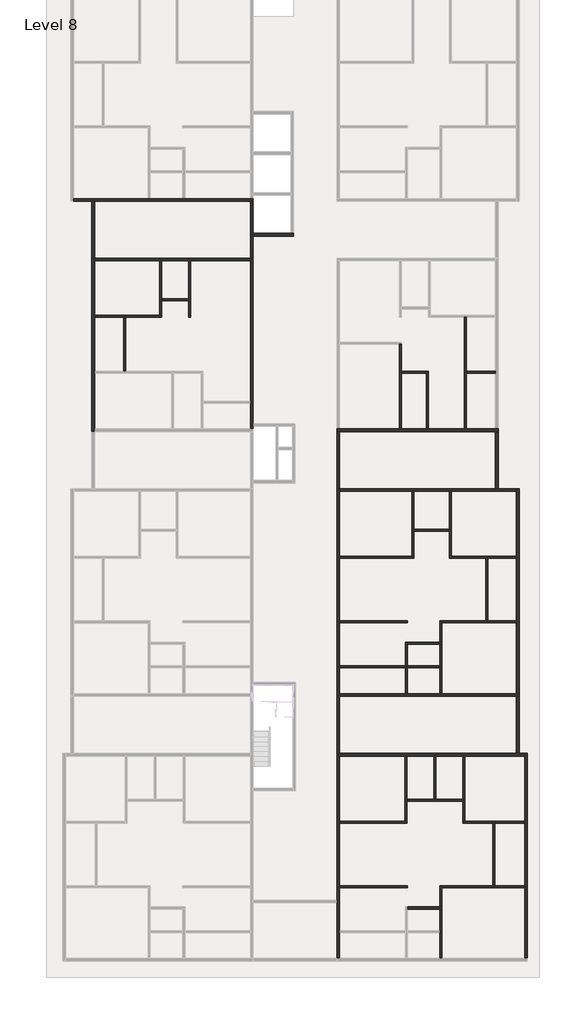
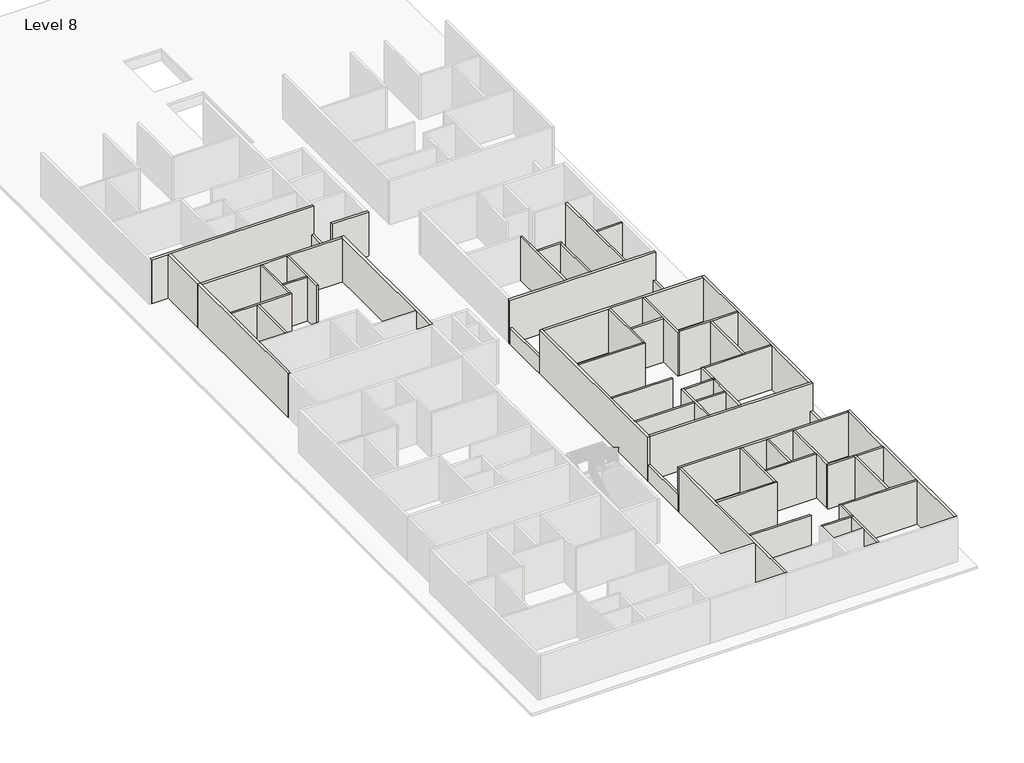
# One storey, part 2 of 8: 56 walls.
"""IFC4 building model written with IfcOpenShell, lengths in millimetres."""

from ifc_helpers import new_model, si_unit, frame, origin, place, context, project, spatial, polyline, outline, extrude, faceted_brep, element, save

model = new_model("IFC4")

# Units and contexts
model_context = context("Model", 3, world=origin())
ifc_project = project(units=[si_unit("LENGTHUNIT", "METRE", prefix="MILLI")], contexts=[model_context])

# Site, building, storey
site = spatial("IfcSite", under=ifc_project)
building = spatial("IfcBuilding", under=site)
storey = spatial("IfcBuildingStorey", under=building, Name="Level 8", Elevation=46570.6172466)

# Walls
placement = place(None, origin())
element("IfcWall", 1, ObjectType="4.5\"", at=placement, inside=storey, context=model_context, shape_type="Brep", body=[
    faceted_brep([(-12531.5544854, 2100.0216096, 46570.6172466), (-10907.2415084, 2100.0216096, 46570.6172466), (-10792.9415084, 2100.0216096, 46570.6172466), (-8759.6544854, 2100.0216096, 46570.6172466), (-8759.6544854, 2100.0216096, 49618.6172466), (-10792.9415084, 2100.0216096, 49618.6172466), (-10907.2415084, 2100.0216096, 49618.6172466), (-12531.5544854, 2100.0216096, 49618.6172466), (-12531.5544854, 2214.3216096, 46570.6172466), (-12531.5544854, 2214.3216096, 49618.6172466), (-8873.9544854, 2214.3216096, 49618.6172466), (-8759.6544854, 2214.3216096, 49618.6172466), (-8759.6544854, 2214.3216096, 46570.6172466), (-8873.9544854, 2214.3216096, 46570.6172466)], [[[0, 1, 2, 3, 4, 5, 6, 7]], [[8, 9, 10, 11, 12, 13]], [[3, 2, 1, 0, 8, 13, 12]], [[0, 7, 9, 8]], [[4, 3, 12, 11]], [[7, 6, 5, 4, 11, 10, 9]]]),
])
element("IfcWall", 2, ObjectType="4.5\"", at=placement, inside=storey, context=model_context, shape_type="Brep", body=[
    faceted_brep([(-8759.6544854, 2214.3216096, 46570.6172466), (-8759.6544854, 3014.4216096, 46570.6172466), (-8759.6544854, 3128.7216096, 46570.6172466), (-8759.6544854, 5264.2743917, 46570.6172466), (-8759.6544854, 5264.2743917, 49618.6172466), (-8759.6544854, 3128.7216096, 49618.6172466), (-8759.6544854, 3014.4216096, 49618.6172466), (-8759.6544854, 2214.3216096, 49618.6172466), (-8873.9544854, 2214.3216096, 46570.6172466), (-8873.9544854, 2214.3216096, 49618.6172466), (-8873.9544854, 5264.2743917, 49618.6172466), (-8873.9544854, 5264.2743917, 46570.6172466)], [[[0, 1, 2, 3, 4, 5, 6, 7]], [[8, 9, 10, 11]], [[3, 2, 1, 0, 8, 11]], [[0, 7, 9, 8]], [[4, 3, 11, 10]], [[7, 6, 5, 4, 10, 9]]]),
])
element("IfcWall", 3, ObjectType="4.5\"", at=placement, inside=storey, context=model_context, shape_type="Brep", body=[
    faceted_brep([(-7235.6544854, 5264.2743917, 46570.6172466), (-7235.6544854, 3128.7216096, 46570.6172466), (-7235.6544854, 3014.4216096, 46570.6172466), (-7235.6544854, 2100.0216096, 46570.6172466), (-7235.6544854, 2100.0216096, 49618.6172466), (-7235.6544854, 3014.4216096, 49618.6172466), (-7235.6544854, 3128.7216096, 49618.6172466), (-7235.6544854, 5264.2743917, 49618.6172466), (-7121.3544854, 5264.2743917, 46570.6172466), (-7121.3544854, 5264.2743917, 49618.6172466), (-7121.3544854, 2100.0216096, 49618.6172466), (-7121.3544854, 2100.0216096, 46570.6172466)], [[[0, 1, 2, 3, 4, 5, 6, 7]], [[8, 9, 10, 11]], [[3, 2, 1, 0, 8, 11]], [[4, 3, 11, 10]], [[0, 7, 9, 8]], [[7, 6, 5, 4, 10, 9]]]),
])
element("IfcWall", 4, ObjectType="4.5\"", at=placement, inside=storey, context=model_context, shape_type="SweptSolid", body=[
    extrude(outline(polyline([(-7235.6544854, 3014.4216096), (-8759.6544854, 3014.4216096), (-8759.6544854, 3128.7216096), (-7235.6544854, 3128.7216096), (-7235.6544854, 3014.4216096)])), frame((0.0, 0.0, 46570.6172466), z_axis=(0.0, 0.0, 1.0), x_axis=(1.0, 0.0, 0.0)), (0.0, 0.0, 1.0), 3048.0),
])
element("IfcWall", 5, ObjectType="4.5\"", at=placement, inside=storey, context=model_context, shape_type="SweptSolid", body=[
    extrude(outline(polyline([(-10907.2415084, -947.4344126), (-10907.2415084, 2100.0216096), (-10792.9415084, 2100.0216096), (-10792.9415084, -947.4344126), (-10907.2415084, -947.4344126)])), frame((0.0, 0.0, 46570.6172466), z_axis=(0.0, 0.0, 1.0), x_axis=(1.0, 0.0, 0.0)), (0.0, 0.0, 1.0), 3048.0),
])
element("IfcWall", 6, ObjectType="4.5\"", at=placement, inside=storey, context=model_context, shape_type="Brep", body=[
    faceted_brep([(5056.6584916, -31173.4344126, 46570.6172466), (6885.4584916, -31173.4344126, 46570.6172466), (6999.7584916, -31173.4344126, 46570.6172466), (6999.7584916, -31173.4344126, 49618.6172466), (6885.4584916, -31173.4344126, 49618.6172466), (5056.6584916, -31173.4344126, 49618.6172466), (5056.6584916, -31059.1344126, 46570.6172466), (5056.6584916, -31059.1344126, 49618.6172466), (6885.4584916, -31059.1344126, 49618.6172466), (6999.7584916, -31059.1344126, 49618.6172466), (6999.7584916, -31059.1344126, 46570.6172466), (6885.4584916, -31059.1344126, 46570.6172466)], [[[0, 1, 2, 3, 4, 5]], [[6, 7, 8, 9, 10, 11]], [[2, 1, 0, 6, 11, 10]], [[0, 5, 7, 6]], [[3, 2, 10, 9]], [[5, 4, 3, 9, 8, 7]]]),
])
element("IfcWall", 7, ObjectType="4.5\"", at=placement, inside=storey, context=model_context, shape_type="Brep", body=[
    faceted_brep([(6885.4584916, -31173.4344126, 46570.6172466), (6885.4584916, -32392.6344126, 46570.6172466), (6885.4584916, -32506.9344126, 46570.6172466), (6885.4584916, -33954.7344126, 46570.6172466), (6885.4584916, -33954.7344126, 49618.6172466), (6885.4584916, -32506.9344126, 49618.6172466), (6885.4584916, -32392.6344126, 49618.6172466), (6885.4584916, -31173.4344126, 49618.6172466), (6999.7584916, -31173.4344126, 46570.6172466), (6999.7584916, -31173.4344126, 49618.6172466), (6999.7584916, -33954.7344126, 49618.6172466), (6999.7584916, -33954.7344126, 46570.6172466)], [[[0, 1, 2, 3, 4, 5, 6, 7]], [[8, 9, 10, 11]], [[3, 2, 1, 0, 8, 11]], [[0, 7, 9, 8]], [[4, 3, 11, 10]], [[7, 6, 5, 4, 10, 9]]]),
])
element("IfcWall", 8, ObjectType="4.5\"", at=placement, inside=storey, context=model_context, shape_type="Brep", body=[
    faceted_brep([(6999.7584916, -31059.1344126, 46570.6172466), (6999.7584916, -29966.9344126, 46570.6172466), (6999.7584916, -29852.6344126, 46570.6172466), (6999.7584916, -29852.6344126, 49618.6172466), (6999.7584916, -29966.9344126, 49618.6172466), (6999.7584916, -31059.1344126, 49618.6172466), (6885.4584916, -31059.1344126, 46570.6172466), (6885.4584916, -31059.1344126, 49618.6172466), (6885.4584916, -29852.6344126, 49618.6172466), (6885.4584916, -29852.6344126, 46570.6172466)], [[[0, 1, 2, 3, 4, 5]], [[6, 7, 8, 9]], [[2, 1, 0, 6, 9]], [[0, 5, 7, 6]], [[3, 2, 9, 8]], [[5, 4, 3, 8, 7]]]),
])
element("IfcWall", 9, ObjectType="4.5\"", at=placement, inside=storey, context=model_context, shape_type="Brep", body=[
    faceted_brep([(6999.7584916, -29966.9344126, 46570.6172466), (11660.6584916, -29966.9344126, 46570.6172466), (11660.6584916, -29966.9344126, 49618.6172466), (6999.7584916, -29966.9344126, 49618.6172466), (6999.7584916, -29852.6344126, 46570.6172466), (6999.7584916, -29852.6344126, 49618.6172466), (9869.9584916, -29852.6344126, 49618.6172466), (9984.2584916, -29852.6344126, 49618.6172466), (11660.6584916, -29852.6344126, 49618.6172466), (11660.6584916, -29852.6344126, 46570.6172466), (9984.2584916, -29852.6344126, 46570.6172466), (9869.9584916, -29852.6344126, 46570.6172466)], [[[0, 1, 2, 3]], [[4, 5, 6, 7, 8, 9, 10, 11]], [[1, 0, 4, 11, 10, 9]], [[0, 3, 5, 4]], [[2, 1, 9, 8]], [[3, 2, 8, 7, 6, 5]]]),
])
element("IfcWall", 10, ObjectType="4.5\"", at=placement, inside=storey, context=model_context, shape_type="SweptSolid", body=[
    extrude(outline(polyline([(5056.6584916, -29966.9344126), (1259.3584916, -29966.9344126), (1259.3584916, -29852.6344126), (5056.6584916, -29852.6344126), (5056.6584916, -29966.9344126)])), frame((0.0, 0.0, 46570.6172466), z_axis=(0.0, 0.0, 1.0), x_axis=(1.0, 0.0, 0.0)), (0.0, 0.0, 1.0), 3048.0),
])
element("IfcWall", 11, ObjectType="4.5\"", at=placement, inside=storey, context=model_context, shape_type="Brep", body=[
    faceted_brep([(1259.3584916, -26347.4344126, 46570.6172466), (5031.2584916, -26347.4344126, 46570.6172466), (5031.2584916, -26347.4344126, 49618.6172466), (1259.3584916, -26347.4344126, 49618.6172466), (1259.3584916, -26233.1344126, 46570.6172466), (1259.3584916, -26233.1344126, 49618.6172466), (4916.9584916, -26233.1344126, 49618.6172466), (5031.2584916, -26233.1344126, 49618.6172466), (5031.2584916, -26233.1344126, 46570.6172466), (4916.9584916, -26233.1344126, 46570.6172466)], [[[0, 1, 2, 3]], [[4, 5, 6, 7, 8, 9]], [[1, 0, 4, 9, 8]], [[0, 3, 5, 4]], [[2, 1, 8, 7]], [[3, 2, 7, 6, 5]]]),
])
element("IfcWall", 12, ObjectType="4.5\"", at=placement, inside=storey, context=model_context, shape_type="Brep", body=[
    faceted_brep([(5031.2584916, -26233.1344126, 46570.6172466), (5031.2584916, -25128.2344126, 46570.6172466), (5031.2584916, -25013.9344126, 46570.6172466), (5031.2584916, -22575.5344126, 46570.6172466), (5031.2584916, -22575.5344126, 49618.6172466), (5031.2584916, -25013.9344126, 49618.6172466), (5031.2584916, -25128.2344126, 49618.6172466), (5031.2584916, -26233.1344126, 49618.6172466), (4916.9584916, -26233.1344126, 46570.6172466), (4916.9584916, -26233.1344126, 49618.6172466), (4916.9584916, -22575.5344126, 49618.6172466), (4916.9584916, -22575.5344126, 46570.6172466)], [[[0, 1, 2, 3, 4, 5, 6, 7]], [[8, 9, 10, 11]], [[3, 2, 1, 0, 8, 11]], [[0, 7, 9, 8]], [[4, 3, 11, 10]], [[7, 6, 5, 4, 10, 9]]]),
])
element("IfcWall", 13, ObjectType="4.5\"", at=placement, inside=storey, context=model_context, shape_type="Brep", body=[
    faceted_brep([(9984.2584916, -29852.6344126, 46570.6172466), (9984.2584916, -26347.4344126, 46570.6172466), (9984.2584916, -26233.1344126, 46570.6172466), (9984.2584916, -26233.1344126, 49618.6172466), (9984.2584916, -26347.4344126, 49618.6172466), (9984.2584916, -29852.6344126, 49618.6172466), (9869.9584916, -29852.6344126, 46570.6172466), (9869.9584916, -29852.6344126, 49618.6172466), (9869.9584916, -26347.4344126, 49618.6172466), (9869.9584916, -26233.1344126, 49618.6172466), (9869.9584916, -26233.1344126, 46570.6172466), (9869.9584916, -26347.4344126, 46570.6172466)], [[[0, 1, 2, 3, 4, 5]], [[6, 7, 8, 9, 10, 11]], [[2, 1, 0, 6, 11, 10]], [[0, 5, 7, 6]], [[3, 2, 10, 9]], [[5, 4, 3, 9, 8, 7]]]),
])
element("IfcWall", 14, ObjectType="4.5\"", at=placement, inside=storey, context=model_context, shape_type="SweptSolid", body=[
    extrude(outline(polyline([(11660.6584916, -26347.4344126), (9984.2584916, -26347.4344126), (9984.2584916, -26233.1344126), (11660.6584916, -26233.1344126), (11660.6584916, -26347.4344126)])), frame((0.0, 0.0, 46570.6172466), z_axis=(0.0, 0.0, 1.0), x_axis=(1.0, 0.0, 0.0)), (0.0, 0.0, 1.0), 3048.0),
])
element("IfcWall", 15, ObjectType="4.5\"", at=placement, inside=storey, context=model_context, shape_type="Brep", body=[
    faceted_brep([(9869.9584916, -26233.1344126, 46570.6172466), (8307.8584916, -26233.1344126, 46570.6172466), (8193.5584916, -26233.1344126, 46570.6172466), (8193.5584916, -26233.1344126, 49618.6172466), (8307.8584916, -26233.1344126, 49618.6172466), (9869.9584916, -26233.1344126, 49618.6172466), (9869.9584916, -26347.4344126, 46570.6172466), (9869.9584916, -26347.4344126, 49618.6172466), (8193.5584916, -26347.4344126, 49618.6172466), (8193.5584916, -26347.4344126, 46570.6172466)], [[[0, 1, 2, 3, 4, 5]], [[6, 7, 8, 9]], [[2, 1, 0, 6, 9]], [[0, 5, 7, 6]], [[3, 2, 9, 8]], [[5, 4, 3, 8, 7]]]),
])
element("IfcWall", 16, ObjectType="4.5\"", at=placement, inside=storey, context=model_context, shape_type="Brep", body=[
    faceted_brep([(8307.8584916, -26233.1344126, 46570.6172466), (8307.8584916, -22575.5344126, 46570.6172466), (8307.8584916, -22575.5344126, 49618.6172466), (8307.8584916, -26233.1344126, 49618.6172466), (8193.5584916, -26233.1344126, 46570.6172466), (8193.5584916, -26233.1344126, 49618.6172466), (8193.5584916, -25128.2344126, 49618.6172466), (8193.5584916, -25013.9344126, 49618.6172466), (8193.5584916, -22575.5344126, 49618.6172466), (8193.5584916, -22575.5344126, 46570.6172466), (8193.5584916, -25013.9344126, 46570.6172466), (8193.5584916, -25128.2344126, 46570.6172466)], [[[0, 1, 2, 3]], [[4, 5, 6, 7, 8, 9, 10, 11]], [[1, 0, 4, 11, 10, 9]], [[0, 3, 5, 4]], [[2, 1, 9, 8]], [[3, 2, 8, 7, 6, 5]]]),
])
element("IfcWall", 17, ObjectType="4.5\"", at=placement, inside=storey, context=model_context, shape_type="Brep", body=[
    faceted_brep([(5031.2584916, -25128.2344126, 46570.6172466), (8193.5584916, -25128.2344126, 46570.6172466), (8193.5584916, -25128.2344126, 49618.6172466), (5031.2584916, -25128.2344126, 49618.6172466), (5031.2584916, -25013.9344126, 46570.6172466), (5031.2584916, -25013.9344126, 49618.6172466), (6555.2584916, -25013.9344126, 49618.6172466), (6669.5584916, -25013.9344126, 49618.6172466), (8193.5584916, -25013.9344126, 49618.6172466), (8193.5584916, -25013.9344126, 46570.6172466), (6669.5584916, -25013.9344126, 46570.6172466), (6555.2584916, -25013.9344126, 46570.6172466)], [[[0, 1, 2, 3]], [[4, 5, 6, 7, 8, 9, 10, 11]], [[1, 0, 4, 11, 10, 9]], [[0, 3, 5, 4]], [[2, 1, 9, 8]], [[3, 2, 8, 7, 6, 5]]]),
])
element("IfcWall", 18, ObjectType="4.5\"", at=placement, inside=storey, context=model_context, shape_type="SweptSolid", body=[
    extrude(outline(polyline([(6555.2584916, -25013.9344126), (6555.2584916, -22575.5344126), (6669.5584916, -22575.5344126), (6669.5584916, -25013.9344126), (6555.2584916, -25013.9344126)])), frame((0.0, 0.0, 46570.6172466), z_axis=(0.0, 0.0, 1.0), x_axis=(1.0, 0.0, 0.0)), (0.0, 0.0, 1.0), 3048.0),
])
element("IfcWall", 19, ObjectType="4.5\"", at=placement, inside=storey, context=model_context, shape_type="SweptSolid", body=[
    extrude(outline(polyline([(4942.3584916, -17622.5344126), (1259.3584916, -17622.5344126), (1259.3584916, -17508.2344126), (4942.3584916, -17508.2344126), (4942.3584916, -17622.5344126)])), frame((0.0, 0.0, 46570.6172466), z_axis=(0.0, 0.0, 1.0), x_axis=(1.0, 0.0, 0.0)), (0.0, 0.0, 1.0), 3048.0),
])
element("IfcWall", 20, ObjectType="4.5\"", at=placement, inside=storey, context=model_context, shape_type="Brep", body=[
    faceted_brep([(4942.3584916, -16174.7344126, 46570.6172466), (4942.3584916, -17508.2344126, 46570.6172466), (4942.3584916, -17622.5344126, 46570.6172466), (4942.3584916, -19070.3344126, 46570.6172466), (4942.3584916, -19070.3344126, 49618.6172466), (4942.3584916, -17622.5344126, 49618.6172466), (4942.3584916, -17508.2344126, 49618.6172466), (4942.3584916, -16174.7344126, 49618.6172466), (5056.6584916, -16174.7344126, 46570.6172466), (5056.6584916, -16174.7344126, 49618.6172466), (5056.6584916, -16289.0344126, 49618.6172466), (5056.6584916, -17508.2344126, 49618.6172466), (5056.6584916, -17622.5344126, 49618.6172466), (5056.6584916, -19070.3344126, 49618.6172466), (5056.6584916, -19070.3344126, 46570.6172466), (5056.6584916, -17622.5344126, 46570.6172466), (5056.6584916, -17508.2344126, 46570.6172466), (5056.6584916, -16289.0344126, 46570.6172466)], [[[0, 1, 2, 3, 4, 5, 6, 7]], [[8, 9, 10, 11, 12, 13, 14, 15, 16, 17]], [[3, 2, 1, 0, 8, 17, 16, 15, 14]], [[4, 3, 14, 13]], [[0, 7, 9, 8]], [[7, 6, 5, 4, 13, 12, 11, 10, 9]]]),
])
element("IfcWall", 21, ObjectType="4.5\"", at=placement, inside=storey, context=model_context, shape_type="Brep", body=[
    faceted_brep([(5056.6584916, -16289.0344126, 46570.6172466), (6885.4584916, -16289.0344126, 46570.6172466), (6999.7584916, -16289.0344126, 46570.6172466), (6999.7584916, -16289.0344126, 49618.6172466), (6885.4584916, -16289.0344126, 49618.6172466), (5056.6584916, -16289.0344126, 49618.6172466), (5056.6584916, -16174.7344126, 46570.6172466), (5056.6584916, -16174.7344126, 49618.6172466), (6885.4584916, -16174.7344126, 49618.6172466), (6999.7584916, -16174.7344126, 49618.6172466), (6999.7584916, -16174.7344126, 46570.6172466), (6885.4584916, -16174.7344126, 46570.6172466)], [[[0, 1, 2, 3, 4, 5]], [[6, 7, 8, 9, 10, 11]], [[2, 1, 0, 6, 11, 10]], [[0, 5, 7, 6]], [[3, 2, 10, 9]], [[5, 4, 3, 9, 8, 7]]]),
])
element("IfcWall", 22, ObjectType="4.5\"", at=placement, inside=storey, context=model_context, shape_type="Brep", body=[
    faceted_brep([(6885.4584916, -16289.0344126, 46570.6172466), (6885.4584916, -17508.2344126, 46570.6172466), (6885.4584916, -17622.5344126, 46570.6172466), (6885.4584916, -19070.3344126, 46570.6172466), (6885.4584916, -19070.3344126, 49618.6172466), (6885.4584916, -17622.5344126, 49618.6172466), (6885.4584916, -17508.2344126, 49618.6172466), (6885.4584916, -16289.0344126, 49618.6172466), (6999.7584916, -16289.0344126, 46570.6172466), (6999.7584916, -16289.0344126, 49618.6172466), (6999.7584916, -19070.3344126, 49618.6172466), (6999.7584916, -19070.3344126, 46570.6172466)], [[[0, 1, 2, 3, 4, 5, 6, 7]], [[8, 9, 10, 11]], [[3, 2, 1, 0, 8, 11]], [[0, 7, 9, 8]], [[4, 3, 11, 10]], [[7, 6, 5, 4, 10, 9]]]),
])
element("IfcWall", 23, ObjectType="4.5\"", at=placement, inside=storey, context=model_context, shape_type="SweptSolid", body=[
    extrude(outline(polyline([(6885.4584916, -17622.5344126), (5056.6584916, -17622.5344126), (5056.6584916, -17508.2344126), (6885.4584916, -17508.2344126), (6885.4584916, -17622.5344126)])), frame((0.0, 0.0, 46570.6172466), z_axis=(0.0, 0.0, 1.0), x_axis=(1.0, 0.0, 0.0)), (0.0, 0.0, 1.0), 3048.0),
])
element("IfcWall", 24, ObjectType="4.5\"", at=placement, inside=storey, context=model_context, shape_type="Brep", body=[
    faceted_brep([(6999.7584916, -16174.7344126, 46570.6172466), (6999.7584916, -15082.5344126, 46570.6172466), (6999.7584916, -14968.2344126, 46570.6172466), (6999.7584916, -14968.2344126, 49618.6172466), (6999.7584916, -15082.5344126, 49618.6172466), (6999.7584916, -16174.7344126, 49618.6172466), (6885.4584916, -16174.7344126, 46570.6172466), (6885.4584916, -16174.7344126, 49618.6172466), (6885.4584916, -14968.2344126, 49618.6172466), (6885.4584916, -14968.2344126, 46570.6172466)], [[[0, 1, 2, 3, 4, 5]], [[6, 7, 8, 9]], [[2, 1, 0, 6, 9]], [[0, 5, 7, 6]], [[3, 2, 9, 8]], [[5, 4, 3, 8, 7]]]),
])
element("IfcWall", 25, ObjectType="4.5\"", at=placement, inside=storey, context=model_context, shape_type="Brep", body=[
    faceted_brep([(6999.7584916, -15082.5344126, 46570.6172466), (11208.5214687, -15082.5344126, 46570.6172466), (11208.5214687, -15082.5344126, 49618.6172466), (6999.7584916, -15082.5344126, 49618.6172466), (6999.7584916, -14968.2344126, 46570.6172466), (6999.7584916, -14968.2344126, 49618.6172466), (9469.9084916, -14968.2344126, 49618.6172466), (9584.2084916, -14968.2344126, 49618.6172466), (11208.5214687, -14968.2344126, 49618.6172466), (11208.5214687, -14968.2344126, 46570.6172466), (9584.2084916, -14968.2344126, 46570.6172466), (9469.9084916, -14968.2344126, 46570.6172466)], [[[0, 1, 2, 3]], [[4, 5, 6, 7, 8, 9, 10, 11]], [[1, 0, 4, 11, 10, 9]], [[0, 3, 5, 4]], [[2, 1, 9, 8]], [[3, 2, 8, 7, 6, 5]]]),
])
element("IfcWall", 26, ObjectType="4.5\"", at=placement, inside=storey, context=model_context, shape_type="SweptSolid", body=[
    extrude(outline(polyline([(5056.6584916, -15082.5344126), (1259.3584916, -15082.5344126), (1259.3584916, -14968.2344126), (5056.6584916, -14968.2344126), (5056.6584916, -15082.5344126)])), frame((0.0, 0.0, 46570.6172466), z_axis=(0.0, 0.0, 1.0), x_axis=(1.0, 0.0, 0.0)), (0.0, 0.0, 1.0), 3048.0),
])
element("IfcWall", 27, ObjectType="4.5\"", at=placement, inside=storey, context=model_context, shape_type="Brep", body=[
    faceted_brep([(1259.3584916, -11463.0344126, 46570.6172466), (5430.0214687, -11463.0344126, 46570.6172466), (5430.0214687, -11463.0344126, 49618.6172466), (1259.3584916, -11463.0344126, 49618.6172466), (1259.3584916, -11348.7344126, 46570.6172466), (1259.3584916, -11348.7344126, 49618.6172466), (5315.7214687, -11348.7344126, 49618.6172466), (5430.0214687, -11348.7344126, 49618.6172466), (5430.0214687, -11348.7344126, 46570.6172466), (5315.7214687, -11348.7344126, 46570.6172466)], [[[0, 1, 2, 3]], [[4, 5, 6, 7, 8, 9]], [[1, 0, 4, 9, 8]], [[0, 3, 5, 4]], [[2, 1, 8, 7]], [[3, 2, 7, 6, 5]]]),
])
element("IfcWall", 28, ObjectType="4.5\"", at=placement, inside=storey, context=model_context, shape_type="Brep", body=[
    faceted_brep([(5430.0214687, -11348.7344126, 46570.6172466), (5430.0214687, -9939.0344126, 46570.6172466), (5430.0214687, -9824.7344126, 46570.6172466), (5430.0214687, -7691.1344126, 46570.6172466), (5430.0214687, -7691.1344126, 49618.6172466), (5430.0214687, -9824.7344126, 49618.6172466), (5430.0214687, -9939.0344126, 49618.6172466), (5430.0214687, -11348.7344126, 49618.6172466), (5315.7214687, -11348.7344126, 46570.6172466), (5315.7214687, -11348.7344126, 49618.6172466), (5315.7214687, -7691.1344126, 49618.6172466), (5315.7214687, -7691.1344126, 46570.6172466)], [[[0, 1, 2, 3, 4, 5, 6, 7]], [[8, 9, 10, 11]], [[3, 2, 1, 0, 8, 11]], [[0, 7, 9, 8]], [[4, 3, 11, 10]], [[7, 6, 5, 4, 10, 9]]]),
])
element("IfcWall", 29, ObjectType="4.5\"", at=placement, inside=storey, context=model_context, shape_type="SweptSolid", body=[
    extrude(outline(polyline([(7436.6214687, -9939.0344126), (5430.0214687, -9939.0344126), (5430.0214687, -9824.7344126), (7436.6214687, -9824.7344126), (7436.6214687, -9939.0344126)])), frame((0.0, 0.0, 46570.6172466), z_axis=(0.0, 0.0, 1.0), x_axis=(1.0, 0.0, 0.0)), (0.0, 0.0, 1.0), 3048.0),
])
element("IfcWall", 30, ObjectType="4.5\"", at=placement, inside=storey, context=model_context, shape_type="Brep", body=[
    faceted_brep([(7436.6214687, -7691.1344126, 46570.6172466), (7436.6214687, -9824.7344126, 46570.6172466), (7436.6214687, -9939.0344126, 46570.6172466), (7436.6214687, -11463.0344126, 46570.6172466), (7436.6214687, -11463.0344126, 49618.6172466), (7436.6214687, -9939.0344126, 49618.6172466), (7436.6214687, -9824.7344126, 49618.6172466), (7436.6214687, -7691.1344126, 49618.6172466), (7550.9214687, -7691.1344126, 46570.6172466), (7550.9214687, -7691.1344126, 49618.6172466), (7550.9214687, -11348.7344126, 49618.6172466), (7550.9214687, -11463.0344126, 49618.6172466), (7550.9214687, -11463.0344126, 46570.6172466), (7550.9214687, -11348.7344126, 46570.6172466)], [[[0, 1, 2, 3, 4, 5, 6, 7]], [[8, 9, 10, 11, 12, 13]], [[3, 2, 1, 0, 8, 13, 12]], [[0, 7, 9, 8]], [[4, 3, 12, 11]], [[7, 6, 5, 4, 11, 10, 9]]]),
])
element("IfcWall", 31, ObjectType="4.5\"", at=placement, inside=storey, context=model_context, shape_type="Brep", body=[
    faceted_brep([(7550.9214687, -11463.0344126, 46570.6172466), (9469.9084916, -11463.0344126, 46570.6172466), (9584.2084916, -11463.0344126, 46570.6172466), (11208.5214687, -11463.0344126, 46570.6172466), (11208.5214687, -11463.0344126, 49618.6172466), (9584.2084916, -11463.0344126, 49618.6172466), (9469.9084916, -11463.0344126, 49618.6172466), (7550.9214687, -11463.0344126, 49618.6172466), (7550.9214687, -11348.7344126, 46570.6172466), (7550.9214687, -11348.7344126, 49618.6172466), (11208.5214687, -11348.7344126, 49618.6172466), (11208.5214687, -11348.7344126, 46570.6172466)], [[[0, 1, 2, 3, 4, 5, 6, 7]], [[8, 9, 10, 11]], [[3, 2, 1, 0, 8, 11]], [[0, 7, 9, 8]], [[4, 3, 11, 10]], [[7, 6, 5, 4, 10, 9]]]),
])
element("IfcWall", 32, ObjectType="4.5\"", at=placement, inside=storey, context=model_context, shape_type="SweptSolid", body=[
    extrude(outline(polyline([(9469.9084916, -14968.2344126), (9469.9084916, -11463.0344126), (9584.2084916, -11463.0344126), (9584.2084916, -14968.2344126), (9469.9084916, -14968.2344126)])), frame((0.0, 0.0, 46570.6172466), z_axis=(0.0, 0.0, 1.0), x_axis=(1.0, 0.0, 0.0)), (0.0, 0.0, 1.0), 3048.0),
])
element("IfcWall", 33, ObjectType="4.5\"", at=placement, inside=storey, context=model_context, shape_type="Brep", body=[
    faceted_brep([(4610.8714687, 572.7745083, 46570.6172466), (4610.8714687, -4185.9344126, 46570.6172466), (4610.8714687, -4185.9344126, 49618.6172466), (4610.8714687, 572.7745083, 49618.6172466), (4725.1714687, 572.7745083, 46570.6172466), (4725.1714687, 572.7745083, 49618.6172466), (4725.1714687, -947.4344126, 49618.6172466), (4725.1714687, -1061.7344126, 49618.6172466), (4725.1714687, -4185.9344126, 49618.6172466), (4725.1714687, -4185.9344126, 46570.6172466), (4725.1714687, -1061.7344126, 46570.6172466), (4725.1714687, -947.4344126, 46570.6172466)], [[[0, 1, 2, 3]], [[4, 5, 6, 7, 8, 9, 10, 11]], [[1, 0, 4, 11, 10, 9]], [[0, 3, 5, 4]], [[2, 1, 9, 8]], [[3, 2, 8, 7, 6, 5]]]),
])
element("IfcWall", 34, ObjectType="4.5\"", at=placement, inside=storey, context=model_context, shape_type="Brep", body=[
    faceted_brep([(4725.1714687, -1061.7344126, 46570.6172466), (6134.8714687, -1061.7344126, 46570.6172466), (6249.1714687, -1061.7344126, 46570.6172466), (6249.1714687, -1061.7344126, 49618.6172466), (6134.8714687, -1061.7344126, 49618.6172466), (4725.1714687, -1061.7344126, 49618.6172466), (4725.1714687, -947.4344126, 46570.6172466), (4725.1714687, -947.4344126, 49618.6172466), (6249.1714687, -947.4344126, 49618.6172466), (6249.1714687, -947.4344126, 46570.6172466)], [[[0, 1, 2, 3, 4, 5]], [[6, 7, 8, 9]], [[2, 1, 0, 6, 9]], [[0, 5, 7, 6]], [[3, 2, 9, 8]], [[5, 4, 3, 8, 7]]]),
])
element("IfcWall", 35, ObjectType="4.5\"", at=placement, inside=storey, context=model_context, shape_type="SweptSolid", body=[
    extrude(outline(polyline([(6134.8714687, -4185.9344126), (6134.8714687, -1061.7344126), (6249.1714687, -1061.7344126), (6249.1714687, -4185.9344126), (6134.8714687, -4185.9344126)])), frame((0.0, 0.0, 46570.6172466), z_axis=(0.0, 0.0, 1.0), x_axis=(1.0, 0.0, 0.0)), (0.0, 0.0, 1.0), 3048.0),
])
element("IfcWall", 36, ObjectType="4.5\"", at=placement, inside=storey, context=model_context, shape_type="Brep", body=[
    faceted_brep([(8396.7584916, -4185.9344126, 46570.6172466), (8396.7584916, -1061.7344126, 46570.6172466), (8396.7584916, -947.4344126, 46570.6172466), (8396.7584916, 2100.0216096, 46570.6172466), (8396.7584916, 2100.0216096, 49618.6172466), (8396.7584916, -947.4344126, 49618.6172466), (8396.7584916, -1061.7344126, 49618.6172466), (8396.7584916, -4185.9344126, 49618.6172466), (8282.4584916, -4185.9344126, 46570.6172466), (8282.4584916, -4185.9344126, 49618.6172466), (8282.4584916, 2100.0216096, 49618.6172466), (8282.4584916, 2100.0216096, 46570.6172466)], [[[0, 1, 2, 3, 4, 5, 6, 7]], [[8, 9, 10, 11]], [[3, 2, 1, 0, 8, 11]], [[0, 7, 9, 8]], [[4, 3, 11, 10]], [[7, 6, 5, 4, 10, 9]]]),
])
element("IfcWall", 37, ObjectType="4.5\"", at=placement, inside=storey, context=model_context, shape_type="SweptSolid", body=[
    extrude(outline(polyline([(8396.7584916, -947.4344126), (10021.0714687, -947.4344126), (10021.0714687, -1061.7344126), (8396.7584916, -1061.7344126), (8396.7584916, -947.4344126)])), frame((0.0, 0.0, 46570.6172466), z_axis=(0.0, 0.0, 1.0), x_axis=(1.0, 0.0, 0.0)), (0.0, 0.0, 1.0), 3048.0),
])
element("IfcWall", 38, ObjectType="6\"", at=placement, inside=storey, context=model_context, shape_type="Brep", body=[
    faceted_brep([(-13719.0044854, 8615.1216096, 46570.6172466), (-12683.9544854, 8615.1216096, 46570.6172466), (-12531.5544854, 8615.1216096, 46570.6172466), (-3769.8415084, 8615.1216096, 46570.6172466), (-3617.4415084, 8615.1216096, 46570.6172466), (-3617.4415084, 8615.1216096, 47789.8172466), (-3617.4415084, 8615.1216096, 49618.6172466), (-12531.5544854, 8615.1216096, 49618.6172466), (-12683.9544854, 8615.1216096, 49618.6172466), (-13719.0044854, 8615.1216096, 49618.6172466), (-13719.0044854, 8767.5216096, 46570.6172466), (-13719.0044854, 8767.5216096, 49618.6172466), (-9510.2415084, 8767.5216096, 49618.6172466), (-9395.9415084, 8767.5216096, 49618.6172466), (-7567.1415084, 8767.5216096, 49618.6172466), (-7452.8415084, 8767.5216096, 49618.6172466), (-3769.8415084, 8767.5216096, 49618.6172466), (-3617.4415084, 8767.5216096, 49618.6172466), (-3617.4415084, 8767.5216096, 46570.6172466), (-3769.8415084, 8767.5216096, 46570.6172466), (-7452.8415084, 8767.5216096, 46570.6172466), (-7567.1415084, 8767.5216096, 46570.6172466), (-9395.9415084, 8767.5216096, 46570.6172466), (-9510.2415084, 8767.5216096, 46570.6172466)], [[[0, 1, 2, 3, 4, 5, 6, 7, 8, 9]], [[10, 11, 12, 13, 14, 15, 16, 17, 18, 19, 20, 21, 22, 23]], [[4, 3, 2, 1, 0, 10, 23, 22, 21, 20, 19, 18]], [[0, 9, 11, 10]], [[4, 18, 17, 6, 5]], [[9, 8, 7, 6, 17, 16, 15, 14, 13, 12, 11]]]),
])
element("IfcWall", 39, ObjectType="6\"", at=placement, inside=storey, context=model_context, shape_type="Brep", body=[
    faceted_brep([(-12683.9544854, 5416.6743917, 46570.6172466), (-12683.9544854, -4338.3344126, 46570.6172466), (-12683.9544854, -4338.3344126, 49618.6172466), (-12683.9544854, 5416.6743917, 49618.6172466), (-12531.5544854, 5416.6743917, 46570.6172466), (-12531.5544854, 5416.6743917, 49618.6172466), (-12531.5544854, 5264.2743917, 49618.6172466), (-12531.5544854, 2214.3216096, 49618.6172466), (-12531.5544854, 2100.0216096, 49618.6172466), (-12531.5544854, -947.4344126, 49618.6172466), (-12531.5544854, -1061.7344126, 49618.6172466), (-12531.5544854, -4185.9344126, 49618.6172466), (-12531.5544854, -4338.3344126, 49618.6172466), (-12531.5544854, -4338.3344126, 46570.6172466), (-12531.5544854, -4185.9344126, 46570.6172466), (-12531.5544854, -1061.7344126, 46570.6172466), (-12531.5544854, -947.4344126, 46570.6172466), (-12531.5544854, 2100.0216096, 46570.6172466), (-12531.5544854, 2214.3216096, 46570.6172466), (-12531.5544854, 5264.2743917, 46570.6172466)], [[[0, 1, 2, 3]], [[4, 5, 6, 7, 8, 9, 10, 11, 12, 13, 14, 15, 16, 17, 18, 19]], [[1, 0, 4, 19, 18, 17, 16, 15, 14, 13]], [[2, 1, 13, 12]], [[0, 3, 5, 4]], [[3, 2, 12, 11, 10, 9, 8, 7, 6, 5]]]),
])
element("IfcWall", 40, ObjectType="6\"", at=placement, inside=storey, context=model_context, shape_type="Brep", body=[
    faceted_brep([(-3617.4415084, -4185.9344126, 46570.6172466), (-3617.4415084, -4034.6751812, 46570.6172466), (-3617.4415084, -3882.2751812, 46570.6172466), (-3617.4415084, 5416.6743917, 46570.6172466), (-3617.4415084, 5416.6743917, 49618.6172466), (-3617.4415084, -3882.2751812, 49618.6172466), (-3617.4415084, -4034.6751812, 49618.6172466), (-3617.4415084, -4185.9344126, 49618.6172466), (-3769.8415084, -4185.9344126, 46570.6172466), (-3769.8415084, -4185.9344126, 49618.6172466), (-3769.8415084, -2738.1344126, 49618.6172466), (-3769.8415084, -2623.8344126, 49618.6172466), (-3769.8415084, 5264.2743917, 49618.6172466), (-3769.8415084, 5416.6743917, 49618.6172466), (-3769.8415084, 5416.6743917, 46570.6172466), (-3769.8415084, 5264.2743917, 46570.6172466), (-3769.8415084, -2623.8344126, 46570.6172466), (-3769.8415084, -2738.1344126, 46570.6172466)], [[[0, 1, 2, 3, 4, 5, 6, 7]], [[8, 9, 10, 11, 12, 13, 14, 15, 16, 17]], [[3, 2, 1, 0, 8, 17, 16, 15, 14]], [[0, 7, 9, 8]], [[3, 14, 13, 4]], [[7, 6, 5, 4, 13, 12, 11, 10, 9]]]),
])
element("IfcWall", 41, ObjectType="6\"", at=placement, inside=storey, context=model_context, shape_type="Brep", body=[
    faceted_brep([(-3769.8415084, 5416.6743917, 49618.6172466), (-3769.8415084, 5416.6743917, 46570.6172466), (-12531.5544854, 5416.6743917, 46570.6172466), (-12531.5544854, 5416.6743917, 49618.6172466), (-3769.8415084, 5264.2743917, 46570.6172466), (-3769.8415084, 5264.2743917, 49618.6172466), (-7121.3544854, 5264.2743917, 49618.6172466), (-7235.6544854, 5264.2743917, 49618.6172466), (-8759.6544854, 5264.2743917, 49618.6172466), (-8873.9544854, 5264.2743917, 49618.6172466), (-12531.5544854, 5264.2743917, 49618.6172466), (-12531.5544854, 5264.2743917, 46570.6172466), (-8873.9544854, 5264.2743917, 46570.6172466), (-8759.6544854, 5264.2743917, 46570.6172466), (-7235.6544854, 5264.2743917, 46570.6172466), (-7121.3544854, 5264.2743917, 46570.6172466)], [[[0, 1, 2, 3]], [[4, 5, 6, 7, 8, 9, 10, 11, 12, 13, 14, 15]], [[2, 1, 4, 15, 14, 13, 12, 11]], [[3, 2, 11, 10]], [[0, 5, 4, 1]], [[0, 3, 10, 9, 8, 7, 6, 5]]]),
])
element("IfcWall", 42, ObjectType="6\"", at=placement, inside=storey, context=model_context, shape_type="Brep", body=[
    faceted_brep([(11813.0584916, -33954.7344126, 46570.6172466), (11813.0584916, -22423.1344126, 46570.6172466), (11813.0584916, -22423.1344126, 49618.6172466), (11813.0584916, -33954.7344126, 49618.6172466), (11660.6584916, -33954.7344126, 46570.6172466), (11660.6584916, -33954.7344126, 49618.6172466), (11660.6584916, -29966.9344126, 49618.6172466), (11660.6584916, -29852.6344126, 49618.6172466), (11660.6584916, -26347.4344126, 49618.6172466), (11660.6584916, -26233.1344126, 49618.6172466), (11660.6584916, -22575.5344126, 49618.6172466), (11660.6584916, -22423.1344126, 49618.6172466), (11660.6584916, -22423.1344126, 46570.6172466), (11660.6584916, -22575.5344126, 46570.6172466), (11660.6584916, -26233.1344126, 46570.6172466), (11660.6584916, -26347.4344126, 46570.6172466), (11660.6584916, -29852.6344126, 46570.6172466), (11660.6584916, -29966.9344126, 46570.6172466)], [[[0, 1, 2, 3]], [[4, 5, 6, 7, 8, 9, 10, 11, 12, 13, 14, 15, 16, 17]], [[1, 0, 4, 17, 16, 15, 14, 13, 12]], [[0, 3, 5, 4]], [[2, 1, 12, 11]], [[3, 2, 11, 10, 9, 8, 7, 6, 5]]]),
])
element("IfcWall", 43, ObjectType="6\"", at=placement, inside=storey, context=model_context, shape_type="Brep", body=[
    faceted_brep([(11660.6584916, -22423.1344126, 46570.6172466), (11360.9214687, -22423.1344126, 46570.6172466), (11208.5214687, -22423.1344126, 46570.6172466), (1259.3584916, -22423.1344126, 46570.6172466), (1106.9584916, -22423.1344126, 46570.6172466), (1106.9584916, -22423.1344126, 47789.8172466), (1106.9584916, -22423.1344126, 49618.6172466), (11660.6584916, -22423.1344126, 49618.6172466), (11660.6584916, -22575.5344126, 46570.6172466), (11660.6584916, -22575.5344126, 49618.6172466), (8307.8584916, -22575.5344126, 49618.6172466), (8193.5584916, -22575.5344126, 49618.6172466), (6669.5584916, -22575.5344126, 49618.6172466), (6555.2584916, -22575.5344126, 49618.6172466), (5031.2584916, -22575.5344126, 49618.6172466), (4916.9584916, -22575.5344126, 49618.6172466), (1259.3584916, -22575.5344126, 49618.6172466), (1106.9584916, -22575.5344126, 49618.6172466), (1106.9584916, -22575.5344126, 46570.6172466), (1259.3584916, -22575.5344126, 46570.6172466), (4916.9584916, -22575.5344126, 46570.6172466), (5031.2584916, -22575.5344126, 46570.6172466), (6555.2584916, -22575.5344126, 46570.6172466), (6669.5584916, -22575.5344126, 46570.6172466), (8193.5584916, -22575.5344126, 46570.6172466), (8307.8584916, -22575.5344126, 46570.6172466)], [[[0, 1, 2, 3, 4, 5, 6, 7]], [[8, 9, 10, 11, 12, 13, 14, 15, 16, 17, 18, 19, 20, 21, 22, 23, 24, 25]], [[4, 3, 2, 1, 0, 8, 25, 24, 23, 22, 21, 20, 19, 18]], [[0, 7, 9, 8]], [[4, 18, 17, 6, 5]], [[7, 6, 17, 16, 15, 14, 13, 12, 11, 10, 9]]]),
])
element("IfcWall", 44, ObjectType="6\"", at=placement, inside=storey, context=model_context, shape_type="Brep", body=[
    faceted_brep([(1106.9584916, -22575.5344126, 49618.6172466), (1106.9584916, -22575.5344126, 46570.6172466), (1106.9584916, -30668.5325185, 46570.6172466), (1106.9584916, -30820.9325185, 46570.6172466), (1106.9584916, -33954.7344126, 46570.6172466), (1106.9584916, -33954.7344126, 49618.6172466), (1106.9584916, -30820.9325185, 49618.6172466), (1106.9584916, -30668.5325185, 49618.6172466), (1259.3584916, -22575.5344126, 46570.6172466), (1259.3584916, -22575.5344126, 49618.6172466), (1259.3584916, -26233.1344126, 49618.6172466), (1259.3584916, -26347.4344126, 49618.6172466), (1259.3584916, -29852.6344126, 49618.6172466), (1259.3584916, -29966.9344126, 49618.6172466), (1259.3584916, -32392.6344126, 49618.6172466), (1259.3584916, -32506.9344126, 49618.6172466), (1259.3584916, -33954.7344126, 49618.6172466), (1259.3584916, -33954.7344126, 46570.6172466), (1259.3584916, -32506.9344126, 46570.6172466), (1259.3584916, -32392.6344126, 46570.6172466), (1259.3584916, -29966.9344126, 46570.6172466), (1259.3584916, -29852.6344126, 46570.6172466), (1259.3584916, -26347.4344126, 46570.6172466), (1259.3584916, -26233.1344126, 46570.6172466)], [[[0, 1, 2, 3, 4, 5, 6, 7]], [[8, 9, 10, 11, 12, 13, 14, 15, 16, 17, 18, 19, 20, 21, 22, 23]], [[4, 3, 2, 1, 8, 23, 22, 21, 20, 19, 18, 17]], [[5, 4, 17, 16]], [[0, 9, 8, 1]], [[0, 7, 6, 5, 16, 15, 14, 13, 12, 11, 10, 9]]]),
])
element("IfcWall", 45, ObjectType="6\"", at=placement, inside=storey, context=model_context, shape_type="Brep", body=[
    faceted_brep([(1106.9584916, -7538.7344126, 49618.6172466), (1106.9584916, -7538.7344126, 46570.6172466), (1106.9584916, -19222.7344126, 46570.6172466), (1106.9584916, -19222.7344126, 49618.6172466), (1259.3584916, -7538.7344126, 46570.6172466), (1259.3584916, -7538.7344126, 49618.6172466), (1259.3584916, -7691.1344126, 49618.6172466), (1259.3584916, -11348.7344126, 49618.6172466), (1259.3584916, -11463.0344126, 49618.6172466), (1259.3584916, -14968.2344126, 49618.6172466), (1259.3584916, -15082.5344126, 49618.6172466), (1259.3584916, -17508.2344126, 49618.6172466), (1259.3584916, -17622.5344126, 49618.6172466), (1259.3584916, -19070.3344126, 49618.6172466), (1259.3584916, -19222.7344126, 49618.6172466), (1259.3584916, -19222.7344126, 46570.6172466), (1259.3584916, -19070.3344126, 46570.6172466), (1259.3584916, -17622.5344126, 46570.6172466), (1259.3584916, -17508.2344126, 46570.6172466), (1259.3584916, -15082.5344126, 46570.6172466), (1259.3584916, -14968.2344126, 46570.6172466), (1259.3584916, -11463.0344126, 46570.6172466), (1259.3584916, -11348.7344126, 46570.6172466), (1259.3584916, -7691.1344126, 46570.6172466)], [[[0, 1, 2, 3]], [[4, 5, 6, 7, 8, 9, 10, 11, 12, 13, 14, 15, 16, 17, 18, 19, 20, 21, 22, 23]], [[2, 1, 4, 23, 22, 21, 20, 19, 18, 17, 16, 15]], [[0, 5, 4, 1]], [[2, 15, 14, 3]], [[0, 3, 14, 13, 12, 11, 10, 9, 8, 7, 6, 5]]]),
])
element("IfcWall", 46, ObjectType="6\"", at=placement, inside=storey, context=model_context, shape_type="Brep", body=[
    faceted_brep([(1259.3584916, -19222.7344126, 49618.6172466), (1259.3584916, -19222.7344126, 46570.6172466), (11208.5214687, -19222.7344126, 46570.6172466), (11360.9214687, -19222.7344126, 46570.6172466), (11360.9214687, -19222.7344126, 47789.8172466), (11360.9214687, -19222.7344126, 49618.6172466), (1259.3584916, -19070.3344126, 46570.6172466), (1259.3584916, -19070.3344126, 49618.6172466), (4942.3584916, -19070.3344126, 49618.6172466), (5056.6584916, -19070.3344126, 49618.6172466), (6885.4584916, -19070.3344126, 49618.6172466), (6999.7584916, -19070.3344126, 49618.6172466), (11208.5214687, -19070.3344126, 49618.6172466), (11360.9214687, -19070.3344126, 49618.6172466), (11360.9214687, -19070.3344126, 46570.6172466), (11208.5214687, -19070.3344126, 46570.6172466), (6999.7584916, -19070.3344126, 46570.6172466), (6885.4584916, -19070.3344126, 46570.6172466), (5056.6584916, -19070.3344126, 46570.6172466), (4942.3584916, -19070.3344126, 46570.6172466)], [[[0, 1, 2, 3, 4, 5]], [[6, 7, 8, 9, 10, 11, 12, 13, 14, 15, 16, 17, 18, 19]], [[3, 2, 1, 6, 19, 18, 17, 16, 15, 14]], [[3, 14, 13, 5, 4]], [[0, 7, 6, 1]], [[0, 5, 13, 12, 11, 10, 9, 8, 7]]]),
])
element("IfcWall", 47, ObjectType="6\"", at=placement, inside=storey, context=model_context, shape_type="Brep", body=[
    faceted_brep([(11360.9214687, -19070.3344126, 49618.6172466), (11360.9214687, -19070.3344126, 46570.6172466), (11360.9214687, -7538.7344126, 46570.6172466), (11360.9214687, -7538.7344126, 49618.6172466), (11208.5214687, -19070.3344126, 46570.6172466), (11208.5214687, -19070.3344126, 49618.6172466), (11208.5214687, -15082.5344126, 49618.6172466), (11208.5214687, -14968.2344126, 49618.6172466), (11208.5214687, -11463.0344126, 49618.6172466), (11208.5214687, -11348.7344126, 49618.6172466), (11208.5214687, -7691.1344126, 49618.6172466), (11208.5214687, -7538.7344126, 49618.6172466), (11208.5214687, -7538.7344126, 46570.6172466), (11208.5214687, -7691.1344126, 46570.6172466), (11208.5214687, -11348.7344126, 46570.6172466), (11208.5214687, -11463.0344126, 46570.6172466), (11208.5214687, -14968.2344126, 46570.6172466), (11208.5214687, -15082.5344126, 46570.6172466)], [[[0, 1, 2, 3]], [[4, 5, 6, 7, 8, 9, 10, 11, 12, 13, 14, 15, 16, 17]], [[2, 1, 4, 17, 16, 15, 14, 13, 12]], [[3, 2, 12, 11]], [[0, 5, 4, 1]], [[0, 3, 11, 10, 9, 8, 7, 6, 5]]]),
])
element("IfcWall", 48, ObjectType="6\"", at=placement, inside=storey, context=model_context, shape_type="Brep", body=[
    faceted_brep([(11208.5214687, -7538.7344126, 46570.6172466), (10173.4714687, -7538.7344126, 46570.6172466), (10021.0714687, -7538.7344126, 46570.6172466), (1259.3584916, -7538.7344126, 46570.6172466), (1259.3584916, -7538.7344126, 49618.6172466), (11208.5214687, -7538.7344126, 49618.6172466), (11208.5214687, -7691.1344126, 46570.6172466), (11208.5214687, -7691.1344126, 49618.6172466), (7550.9214687, -7691.1344126, 49618.6172466), (7436.6214687, -7691.1344126, 49618.6172466), (5430.0214687, -7691.1344126, 49618.6172466), (5315.7214687, -7691.1344126, 49618.6172466), (1259.3584916, -7691.1344126, 49618.6172466), (1259.3584916, -7691.1344126, 46570.6172466), (5315.7214687, -7691.1344126, 46570.6172466), (5430.0214687, -7691.1344126, 46570.6172466), (7436.6214687, -7691.1344126, 46570.6172466), (7550.9214687, -7691.1344126, 46570.6172466)], [[[0, 1, 2, 3, 4, 5]], [[6, 7, 8, 9, 10, 11, 12, 13, 14, 15, 16, 17]], [[3, 2, 1, 0, 6, 17, 16, 15, 14, 13]], [[0, 5, 7, 6]], [[3, 13, 12, 4]], [[5, 4, 12, 11, 10, 9, 8, 7]]]),
])
element("IfcWall", 49, ObjectType="6\"", at=placement, inside=storey, context=model_context, shape_type="Brep", body=[
    faceted_brep([(1106.9584916, -4338.3344126, 49618.6172466), (1106.9584916, -4338.3344126, 47789.8172466), (1106.9584916, -4338.3344126, 46570.6172466), (1259.3584916, -4338.3344126, 46570.6172466), (10021.0714687, -4338.3344126, 46570.6172466), (10173.4714687, -4338.3344126, 46570.6172466), (10173.4714687, -4338.3344126, 47789.8172466), (10173.4714687, -4338.3344126, 49618.6172466), (1106.9584916, -4185.9344126, 46570.6172466), (1106.9584916, -4185.9344126, 49618.6172466), (1259.3584916, -4185.9344126, 49618.6172466), (4610.8714687, -4185.9344126, 49618.6172466), (4725.1714687, -4185.9344126, 49618.6172466), (6134.8714687, -4185.9344126, 49618.6172466), (6249.1714687, -4185.9344126, 49618.6172466), (8282.4584916, -4185.9344126, 49618.6172466), (8396.7584916, -4185.9344126, 49618.6172466), (10021.0714687, -4185.9344126, 49618.6172466), (10173.4714687, -4185.9344126, 49618.6172466), (10173.4714687, -4185.9344126, 46570.6172466), (10021.0714687, -4185.9344126, 46570.6172466), (8396.7584916, -4185.9344126, 46570.6172466), (8282.4584916, -4185.9344126, 46570.6172466), (6249.1714687, -4185.9344126, 46570.6172466), (6134.8714687, -4185.9344126, 46570.6172466), (4725.1714687, -4185.9344126, 46570.6172466), (4610.8714687, -4185.9344126, 46570.6172466), (1259.3584916, -4185.9344126, 46570.6172466)], [[[0, 1, 2, 3, 4, 5, 6, 7]], [[8, 9, 10, 11, 12, 13, 14, 15, 16, 17, 18, 19, 20, 21, 22, 23, 24, 25, 26, 27]], [[5, 4, 3, 2, 8, 27, 26, 25, 24, 23, 22, 21, 20, 19]], [[0, 9, 8, 2, 1]], [[5, 19, 18, 7, 6]], [[0, 7, 18, 17, 16, 15, 14, 13, 12, 11, 10, 9]]]),
])
element("IfcWall", 50, ObjectType="6\"", at=placement, inside=storey, context=model_context, shape_type="Brep", body=[
    faceted_brep([(-3617.4415084, 6659.2303368, 46570.6172466), (-1331.4415084, 6659.2303368, 46570.6172466), (-1331.4415084, 6659.2303368, 49618.6172466), (-3617.4415084, 6659.2303368, 49618.6172466), (-3617.4415084, 6811.6303368, 46570.6172466), (-3617.4415084, 6811.6303368, 49618.6172466), (-1483.8415084, 6811.6303368, 49618.6172466), (-1331.4415084, 6811.6303368, 49618.6172466), (-1331.4415084, 6811.6303368, 46570.6172466), (-1483.8415084, 6811.6303368, 46570.6172466)], [[[0, 1, 2, 3]], [[4, 5, 6, 7, 8, 9]], [[1, 0, 4, 9, 8]], [[3, 2, 7, 6, 5]], [[0, 3, 5, 4]], [[2, 1, 8, 7]]]),
])
element("IfcWall", 51, ObjectType="6\" 2", at=placement, inside=storey, context=model_context, shape_type="SweptSolid", body=[
    extrude(outline(polyline([(-12683.9544854, 5416.6743917), (-12683.9544854, 8615.1216096), (-12531.5544854, 8615.1216096), (-12531.5544854, 5416.6743917), (-12683.9544854, 5416.6743917)])), frame((0.0, 0.0, 46570.6172466), z_axis=(0.0, 0.0, 1.0), x_axis=(1.0, 0.0, 0.0)), (0.0, 0.0, 1.0), 3048.0),
])
element("IfcWall", 52, ObjectType="6\" 2", at=placement, inside=storey, context=model_context, shape_type="Brep", body=[
    faceted_brep([(-3769.8415084, 8615.1216096, 46570.6172466), (-3769.8415084, 5416.6743917, 46570.6172466), (-3769.8415084, 5416.6743917, 47789.8172466), (-3769.8415084, 8615.1216096, 47789.8172466), (-3617.4415084, 8615.1216096, 46570.6172466), (-3617.4415084, 8615.1216096, 47789.8172466), (-3617.4415084, 5416.6743917, 47789.8172466), (-3617.4415084, 5416.6743917, 46570.6172466), (-3617.4415084, 6659.2303368, 46570.6172466), (-3617.4415084, 6811.6303368, 46570.6172466)], [[[0, 1, 2, 3]], [[4, 5, 6, 7, 8, 9]], [[1, 0, 4, 9, 8, 7]], [[3, 2, 6, 5]], [[0, 3, 5, 4]], [[2, 1, 7, 6]]]),
])
element("IfcWall", 53, ObjectType="6\" 2", at=placement, inside=storey, context=model_context, shape_type="SweptSolid", body=[
    extrude(outline(polyline([(1106.9584916, -7538.7344126), (1106.9584916, -4338.3344126), (1259.3584916, -4338.3344126), (1259.3584916, -7538.7344126), (1106.9584916, -7538.7344126)])), frame((0.0, 0.0, 46570.6172466), z_axis=(0.0, 0.0, 1.0), x_axis=(1.0, 0.0, 0.0)), (0.0, 0.0, 1.0), 1219.2),
])
element("IfcWall", 54, ObjectType="6\" 2", at=placement, inside=storey, context=model_context, shape_type="SweptSolid", body=[
    extrude(outline(polyline([(10021.0714687, -7538.7344126), (10021.0714687, -4338.3344126), (10173.4714687, -4338.3344126), (10173.4714687, -7538.7344126), (10021.0714687, -7538.7344126)])), frame((0.0, 0.0, 46570.6172466), z_axis=(0.0, 0.0, 1.0), x_axis=(1.0, 0.0, 0.0)), (0.0, 0.0, 1.0), 1219.2),
])
element("IfcWall", 55, ObjectType="6\" 2", at=placement, inside=storey, context=model_context, shape_type="SweptSolid", body=[
    extrude(outline(polyline([(11208.5214687, -22423.1344126), (11208.5214687, -19222.7344126), (11360.9214687, -19222.7344126), (11360.9214687, -22423.1344126), (11208.5214687, -22423.1344126)])), frame((0.0, 0.0, 46570.6172466), z_axis=(0.0, 0.0, 1.0), x_axis=(1.0, 0.0, 0.0)), (0.0, 0.0, 1.0), 1219.2),
])
element("IfcWall", 56, ObjectType="6\" 2", at=placement, inside=storey, context=model_context, shape_type="SweptSolid", body=[
    extrude(outline(polyline([(1106.9584916, -22423.1344126), (1106.9584916, -19222.7344126), (1259.3584916, -19222.7344126), (1259.3584916, -22423.1344126), (1106.9584916, -22423.1344126)])), frame((0.0, 0.0, 46570.6172466), z_axis=(0.0, 0.0, 1.0), x_axis=(1.0, 0.0, 0.0)), (0.0, 0.0, 1.0), 1219.2),
])

save(model, "model.ifc")

# Revit data of these elements
# Type "4.5\""
#   Assembly Code = "B2010"
#   Layers, outside or top first: 0' - 4 1/2" "WALLS" (function 1)
# Type "6\""
#   Assembly Code = "B2010"
#   Layers, outside or top first: 0' - 6" "WALLS" (function 1)
# Type "6\" 2"
#   Assembly Code = "B2010"
#   Layers, outside or top first: 0' - 6" "4'" (function 1)
# Elements 1, 2, 3, 4, 5, 6, 7, 8, 9, 10, 11, 12, 13, 14, 15, 16, 17, 18, 19, 20, 21, 22, 23, 24, 25, 26, 27, 28, 29, 30, 31, 32, 33, 34, 35, 36, 37 (IfcWall, "4.5\"")
#   Top Offset = 0' - 0"
#   Base Offset = 0' - 0"
#   Unconnected Height = 10' - 0"
#   wall height = 10' - 0"
#   Phase Created = New Construction
#   Base Constraint = Level 8
#   Materials on its faces: "WALLS"
# Elements 38, 39, 40, 41, 42, 43, 44, 45, 46, 47, 48, 49, 50 (IfcWall, "6\"")
#   Top Offset = 0' - 0"
#   Base Offset = 0' - 0"
#   Unconnected Height = 10' - 0"
#   wall height = 10' - 0"
#   Phase Created = New Construction
#   Base Constraint = Level 8
#   Materials on its faces: "WALLS"
# Element 51 (IfcWall, "6\" 2")
#   Top Offset = 0' - 0"
#   Base Offset = 0' - 0"
#   Unconnected Height = 10' - 0"
#   wall height = 10' - 0"
#   Phase Created = New Construction
#   Base Constraint = Level 8
#   Materials on its faces: "4'"
# Elements 52, 53, 54, 55, 56 (IfcWall, "6\" 2")
#   Top Offset = 0' - 0"
#   Base Offset = 0' - 0"
#   Unconnected Height = 4' - 0"
#   wall height = 4' - 0"
#   Phase Created = New Construction
#   Base Constraint = Level 8
#   Materials on its faces: "4'"
# Materials
#   "WALLS": class "Generic", colour RGB 120 120 120, transparency 0, Cost = 0
#   "4'": class "Generic", colour RGB 120 120 120, transparency 0, Cost = 0
